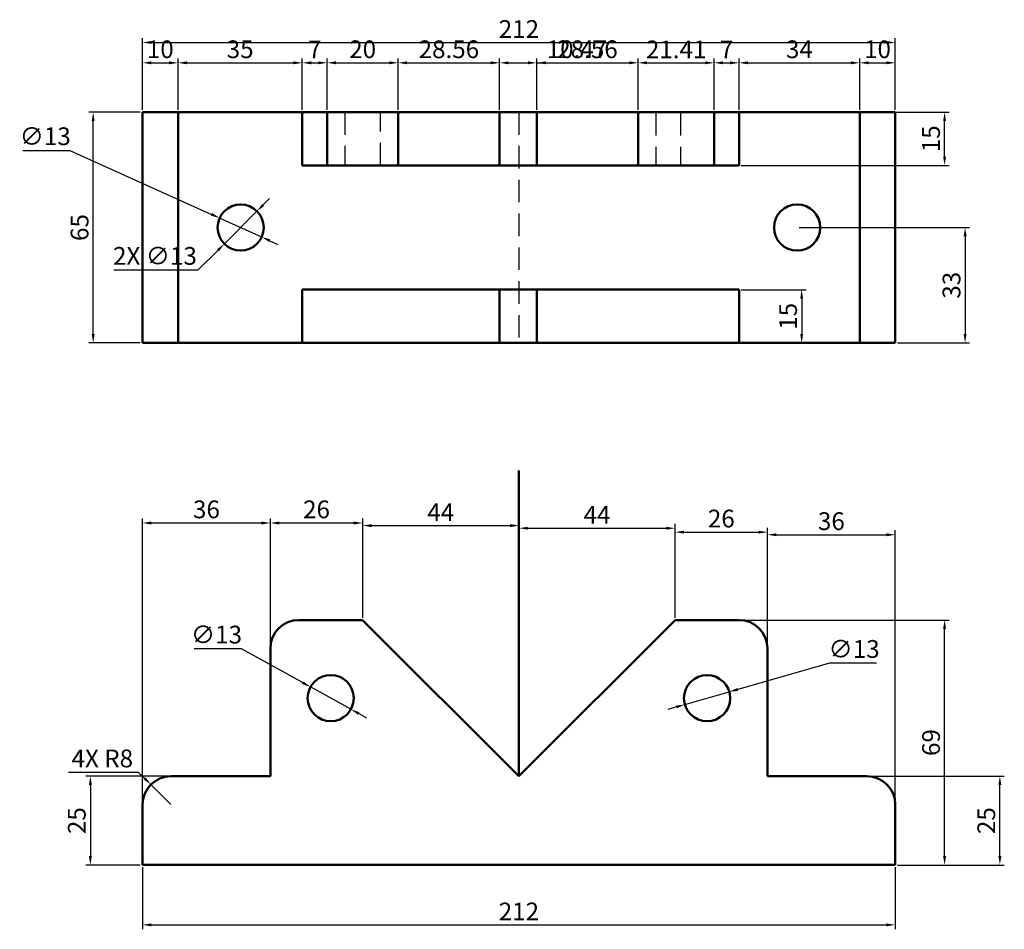
# Model space of a CAD drawing. Units: millimetres. Extents: x 1338 to 1892, y 1867 to 2306.
# Tile 2 of 3: x 1340 to 1617, y 2044 to 2300. Entities that reach past the tile are written whole.
import ezdxf

# ---------------------------------------------------------------- set-up
doc = ezdxf.new("R2010")
doc.units = ezdxf.units.MM
doc.linetypes.add('HIDDEN', pattern=[9.525, 6.35, -3.175])
for name, color, linetype, lineweight in [('M-DIMS', 2, 'Continuous', 25), ('M-HIDN', 4, 'HIDDEN', 25), ('M-OUTL', 7, 'Continuous', 50)]:
    doc.layers.add(name, color=color, linetype=linetype, lineweight=lineweight)
doc.styles.get("Standard").update_dxf_attribs({"font": 'arial.ttf'})
doc.dimstyles.new('ISO-25', dxfattribs={"dimtxt": 5, "dimasz": 2.5, "dimexe": 1.25, "dimexo": 0.625, "dimtad": 1, "dimtoh": 1, "dimdec": 0, "dimtxsty": 'Standard', "dimcen": 2.5, "dimadec": 0, "dimazin": 0, "dimtfac": 1, "dimtdec": 0, "dimtmove": 0, "dimatfit": 3, "dimfxl": 1, "dimarcsym": 0})

# ---------------------------------------------------------------- blocks, each defined once
blk = doc.blocks.new('*D1')
at = {"layer": 'Defpoints', "color": 0, "transparency": 16777216}
for p in [(1586.71, 2293.39), (1374.71, 2273.75), (1586.71, 2273.75)]:
    blk.add_point(p, dxfattribs=at)
at = {"layer": 'M-DIMS', "color": 0, "lineweight": -2, "transparency": 16777216}
for p, q in [((1374.71, 2274.38), (1374.71, 2294.64)), ((1377.21, 2293.39), (1584.21, 2293.39)), ((1586.71, 2274.38), (1586.71, 2294.64))]:
    blk.add_line(p, q, dxfattribs=at)
at = {"layer": 'M-DIMS', "color": 0, "transparency": 16777216}
for points in [[(1377.21, 2293.8), (1377.21, 2292.97), (1374.71, 2293.39)], [(1584.21, 2293.8), (1584.21, 2292.97), (1586.71, 2293.39)]]:
    blk.add_solid(points, dxfattribs=at)
at = {"layer": 'M-DIMS', "color": 0, "transparency": 16777216, "insert": (1480.71, 2296.52), "char_height": 5, "attachment_point": 5}
blk.add_mtext('212', dxfattribs=at)
blk = doc.blocks.new('*D2')
at = {"layer": 'Defpoints', "color": 0, "transparency": 16777216}
for p in [(1559.07, 2241.25), (1586.71, 2208.75), (1606.38, 2208.75)]:
    blk.add_point(p, dxfattribs=at)
at = {"layer": 'M-DIMS', "color": 0, "lineweight": -2, "transparency": 16777216}
for p, q in [((1559.69, 2241.25), (1607.63, 2241.25)), ((1606.38, 2238.75), (1606.38, 2211.25)), ((1587.33, 2208.75), (1607.63, 2208.75))]:
    blk.add_line(p, q, dxfattribs=at)
at = {"layer": 'M-DIMS', "color": 0, "transparency": 16777216}
for points in [[(1605.96, 2238.75), (1606.8, 2238.75), (1606.38, 2241.25)], [(1605.96, 2211.25), (1606.8, 2211.25), (1606.38, 2208.75)]]:
    blk.add_solid(points, dxfattribs=at)
at = {"layer": 'M-DIMS', "color": 0, "transparency": 16777216, "insert": (1603.2, 2225), "char_height": 5, "attachment_point": 5, "rotation": 90}
blk.add_mtext('33', dxfattribs=at)
blk = doc.blocks.new('*D3')
at = {"layer": 'Defpoints', "color": 0, "transparency": 16777216}
for p in [(1396.43, 2243.93), (1408.27, 2238.58)]:
    blk.add_point(p, dxfattribs=at)
at = {"layer": 'M-DIMS', "color": 0, "lineweight": -2, "transparency": 16777216}
for p, q in [((1341.01, 2263), (1354.24, 2263)), ((1354.24, 2263), (1394.15, 2244.96)), ((1408.27, 2238.58), (1396.43, 2243.93)), ((1410.55, 2237.55), (1412.83, 2236.52))]:
    blk.add_line(p, q, dxfattribs=at)
at = {"layer": 'M-DIMS', "color": 0, "transparency": 16777216}
for points in [[(1394.32, 2245.34), (1393.98, 2244.58), (1396.43, 2243.93)], [(1410.72, 2237.93), (1410.38, 2237.17), (1408.27, 2238.58)]]:
    blk.add_solid(points, dxfattribs=at)
at = {"layer": 'M-DIMS', "color": 0, "transparency": 16777216, "insert": (1347.31, 2266.32), "char_height": 5, "attachment_point": 5}
blk.add_mtext('∅13', dxfattribs=at)
blk = doc.blocks.new('*D4')
at = {"layer": 'Defpoints', "color": 0, "transparency": 16777216}
for p in [(1542.71, 2223.75), (1542.71, 2208.75), (1560.35, 2208.75)]:
    blk.add_point(p, dxfattribs=at)
at = {"layer": 'M-DIMS', "color": 0, "lineweight": -2, "transparency": 16777216}
for p, q in [((1543.33, 2223.75), (1561.6, 2223.75)), ((1560.35, 2221.25), (1560.35, 2211.25)), ((1543.33, 2208.75), (1561.6, 2208.75))]:
    blk.add_line(p, q, dxfattribs=at)
at = {"layer": 'M-DIMS', "color": 0, "transparency": 16777216}
for points in [[(1559.93, 2221.25), (1560.77, 2221.25), (1560.35, 2223.75)], [(1559.93, 2211.25), (1560.77, 2211.25), (1560.35, 2208.75)]]:
    blk.add_solid(points, dxfattribs=at)
at = {"layer": 'M-DIMS', "color": 0, "transparency": 16777216, "insert": (1557.17, 2216.25), "char_height": 5, "attachment_point": 5, "rotation": 90}
blk.add_mtext('15', dxfattribs=at)
blk = doc.blocks.new('*D5')
at = {"layer": 'Defpoints', "color": 0, "transparency": 16777216}
for p in [(1374.71, 2061.68), (1586.71, 2061.68), (1586.71, 2044.82)]:
    blk.add_point(p, dxfattribs=at)
at = {"layer": 'M-DIMS', "color": 0, "lineweight": -2, "transparency": 16777216}
for p, q in [((1374.71, 2061.06), (1374.71, 2043.57)), ((1586.71, 2061.06), (1586.71, 2043.57)), ((1377.21, 2044.82), (1584.21, 2044.82))]:
    blk.add_line(p, q, dxfattribs=at)
at = {"layer": 'M-DIMS', "color": 0, "transparency": 16777216}
for points in [[(1377.21, 2045.23), (1377.21, 2044.4), (1374.71, 2044.82)], [(1584.21, 2045.23), (1584.21, 2044.4), (1586.71, 2044.82)]]:
    blk.add_solid(points, dxfattribs=at)
at = {"layer": 'M-DIMS', "color": 0, "transparency": 16777216, "insert": (1480.71, 2047.95), "char_height": 5, "attachment_point": 5}
blk.add_mtext('212', dxfattribs=at)
blk = doc.blocks.new('*D6')
at = {"layer": 'Defpoints', "color": 0, "transparency": 16777216}
for p in [(1382.71, 2086.68), (1360.02, 2061.68), (1374.71, 2061.68)]:
    blk.add_point(p, dxfattribs=at)
at = {"layer": 'M-DIMS', "color": 0, "lineweight": -2, "transparency": 16777216}
for p, q in [((1382.08, 2086.68), (1358.77, 2086.68)), ((1360.02, 2084.18), (1360.02, 2064.18)), ((1374.08, 2061.68), (1358.77, 2061.68))]:
    blk.add_line(p, q, dxfattribs=at)
at = {"layer": 'M-DIMS', "color": 0, "transparency": 16777216}
for points in [[(1359.6, 2084.18), (1360.44, 2084.18), (1360.02, 2086.68)], [(1359.6, 2064.18), (1360.44, 2064.18), (1360.02, 2061.68)]]:
    blk.add_solid(points, dxfattribs=at)
at = {"layer": 'M-DIMS', "color": 0, "transparency": 16777216, "insert": (1356.84, 2074.18), "char_height": 5, "attachment_point": 5, "rotation": 90}
blk.add_mtext('25', dxfattribs=at)
blk = doc.blocks.new('*D7')
at = {"layer": 'Defpoints', "color": 0, "transparency": 16777216}
for p in [(1410.71, 2158.03), (1410.71, 2086.68), (1374.71, 2078.68)]:
    blk.add_point(p, dxfattribs=at)
at = {"layer": 'M-DIMS', "color": 0, "lineweight": -2, "transparency": 16777216}
for p, q in [((1374.71, 2079.31), (1374.71, 2159.28)), ((1377.21, 2158.03), (1408.21, 2158.03)), ((1410.71, 2087.31), (1410.71, 2159.28))]:
    blk.add_line(p, q, dxfattribs=at)
at = {"layer": 'M-DIMS', "color": 0, "transparency": 16777216}
for points in [[(1377.21, 2158.44), (1377.21, 2157.61), (1374.71, 2158.03)], [(1408.21, 2158.44), (1408.21, 2157.61), (1410.71, 2158.03)]]:
    blk.add_solid(points, dxfattribs=at)
at = {"layer": 'M-DIMS', "color": 0, "transparency": 16777216, "insert": (1392.71, 2161.21), "char_height": 5, "attachment_point": 5}
blk.add_mtext('36', dxfattribs=at)
blk = doc.blocks.new('*D8')
at = {"layer": 'Defpoints', "color": 0, "transparency": 16777216}
for p in [(1436.71, 2158.03), (1436.71, 2130.68), (1410.71, 2122.68)]:
    blk.add_point(p, dxfattribs=at)
at = {"layer": 'M-DIMS', "color": 0, "lineweight": -2, "transparency": 16777216}
for p, q in [((1410.71, 2123.31), (1410.71, 2159.28)), ((1413.21, 2158.03), (1434.21, 2158.03)), ((1436.71, 2131.31), (1436.71, 2159.28))]:
    blk.add_line(p, q, dxfattribs=at)
at = {"layer": 'M-DIMS', "color": 0, "transparency": 16777216}
for points in [[(1413.21, 2158.44), (1413.21, 2157.61), (1410.71, 2158.03)], [(1434.21, 2158.44), (1434.21, 2157.61), (1436.71, 2158.03)]]:
    blk.add_solid(points, dxfattribs=at)
at = {"layer": 'M-DIMS', "color": 0, "transparency": 16777216, "insert": (1423.71, 2161.21), "char_height": 5, "attachment_point": 5}
blk.add_mtext('26', dxfattribs=at)
blk = doc.blocks.new('*D9')
at = {"layer": 'Defpoints', "color": 0, "transparency": 16777216}
for p in [(1480.71, 2157.29), (1436.71, 2130.68), (1480.71, 2129.77)]:
    blk.add_point(p, dxfattribs=at)
at = {"layer": 'M-DIMS', "color": 0, "lineweight": -2, "transparency": 16777216}
for p, q in [((1436.71, 2131.31), (1436.71, 2158.54)), ((1480.71, 2130.39), (1480.71, 2158.54)), ((1439.21, 2157.29), (1478.21, 2157.29))]:
    blk.add_line(p, q, dxfattribs=at)
at = {"layer": 'M-DIMS', "color": 0, "transparency": 16777216}
for points in [[(1439.21, 2157.71), (1439.21, 2156.87), (1436.71, 2157.29)], [(1478.21, 2157.71), (1478.21, 2156.87), (1480.71, 2157.29)]]:
    blk.add_solid(points, dxfattribs=at)
at = {"layer": 'M-DIMS', "color": 0, "transparency": 16777216, "insert": (1458.71, 2160.41), "char_height": 5, "attachment_point": 5}
blk.add_mtext('44', dxfattribs=at)
blk = doc.blocks.new('*D10')
at = {"layer": 'Defpoints', "color": 0, "transparency": 16777216}
for p in [(1524.71, 2156.55), (1480.71, 2129.77), (1524.71, 2130.68)]:
    blk.add_point(p, dxfattribs=at)
at = {"layer": 'M-DIMS', "color": 0, "lineweight": -2, "transparency": 16777216}
for p, q in [((1480.71, 2130.39), (1480.71, 2157.8)), ((1524.71, 2131.31), (1524.71, 2157.8)), ((1483.21, 2156.55), (1522.21, 2156.55))]:
    blk.add_line(p, q, dxfattribs=at)
at = {"layer": 'M-DIMS', "color": 0, "transparency": 16777216}
for points in [[(1483.21, 2156.97), (1483.21, 2156.14), (1480.71, 2156.55)], [(1522.21, 2156.97), (1522.21, 2156.14), (1524.71, 2156.55)]]:
    blk.add_solid(points, dxfattribs=at)
at = {"layer": 'M-DIMS', "color": 0, "transparency": 16777216, "insert": (1502.71, 2159.68), "char_height": 5, "attachment_point": 5}
blk.add_mtext('44', dxfattribs=at)
blk = doc.blocks.new('*D11')
at = {"layer": 'Defpoints', "color": 0, "transparency": 16777216}
for p in [(1550.71, 2155.45), (1524.71, 2130.68), (1550.71, 2122.68)]:
    blk.add_point(p, dxfattribs=at)
at = {"layer": 'M-DIMS', "color": 0, "lineweight": -2, "transparency": 16777216}
for p, q in [((1524.71, 2131.31), (1524.71, 2156.7)), ((1527.21, 2155.45), (1548.21, 2155.45)), ((1550.71, 2123.31), (1550.71, 2156.7))]:
    blk.add_line(p, q, dxfattribs=at)
at = {"layer": 'M-DIMS', "color": 0, "transparency": 16777216}
for points in [[(1527.21, 2155.86), (1527.21, 2155.03), (1524.71, 2155.45)], [(1548.21, 2155.86), (1548.21, 2155.03), (1550.71, 2155.45)]]:
    blk.add_solid(points, dxfattribs=at)
at = {"layer": 'M-DIMS', "color": 0, "transparency": 16777216, "insert": (1537.71, 2158.62), "char_height": 5, "attachment_point": 5}
blk.add_mtext('26', dxfattribs=at)
blk = doc.blocks.new('*D12')
at = {"layer": 'Defpoints', "color": 0, "transparency": 16777216}
for p in [(1586.71, 2154.71), (1550.71, 2104.68), (1586.71, 2078.68)]:
    blk.add_point(p, dxfattribs=at)
at = {"layer": 'M-DIMS', "color": 0, "lineweight": -2, "transparency": 16777216}
for p, q in [((1550.71, 2105.31), (1550.71, 2155.96)), ((1553.21, 2154.71), (1584.21, 2154.71)), ((1586.71, 2079.31), (1586.71, 2155.96))]:
    blk.add_line(p, q, dxfattribs=at)
at = {"layer": 'M-DIMS', "color": 0, "transparency": 16777216}
for points in [[(1553.21, 2155.13), (1553.21, 2154.29), (1550.71, 2154.71)], [(1584.21, 2155.13), (1584.21, 2154.29), (1586.71, 2154.71)]]:
    blk.add_solid(points, dxfattribs=at)
at = {"layer": 'M-DIMS', "color": 0, "transparency": 16777216, "insert": (1568.71, 2157.89), "char_height": 5, "attachment_point": 5}
blk.add_mtext('36', dxfattribs=at)
blk = doc.blocks.new('*D13')
at = {"layer": 'Defpoints', "color": 0, "transparency": 16777216}
for p in [(1578.71, 2086.68), (1616.17, 2086.68), (1586.71, 2061.68)]:
    blk.add_point(p, dxfattribs=at)
at = {"layer": 'M-DIMS', "color": 0, "lineweight": -2, "transparency": 16777216}
for p, q in [((1579.33, 2086.68), (1617.42, 2086.68)), ((1616.17, 2064.18), (1616.17, 2084.18)), ((1587.33, 2061.68), (1617.42, 2061.68))]:
    blk.add_line(p, q, dxfattribs=at)
at = {"layer": 'M-DIMS', "color": 0, "transparency": 16777216}
for points in [[(1615.75, 2084.18), (1616.59, 2084.18), (1616.17, 2086.68)], [(1615.75, 2064.18), (1616.59, 2064.18), (1616.17, 2061.68)]]:
    blk.add_solid(points, dxfattribs=at)
at = {"layer": 'M-DIMS', "color": 0, "transparency": 16777216, "insert": (1612.99, 2074.18), "char_height": 5, "attachment_point": 5, "rotation": 90}
blk.add_mtext('25', dxfattribs=at)
blk = doc.blocks.new('*D14')
at = {"layer": 'Defpoints', "color": 0, "transparency": 16777216}
for p in [(1539.96, 2110.47), (1527.46, 2106.89)]:
    blk.add_point(p, dxfattribs=at)
at = {"layer": 'M-DIMS', "color": 0, "lineweight": -2, "transparency": 16777216}
for p, q in [((1568.19, 2118.57), (1542.36, 2111.16)), ((1581.41, 2118.57), (1568.19, 2118.57)), ((1527.46, 2106.89), (1539.96, 2110.47)), ((1525.06, 2106.2), (1522.65, 2105.51))]:
    blk.add_line(p, q, dxfattribs=at)
at = {"layer": 'M-DIMS', "color": 0, "transparency": 16777216}
for points in [[(1542.24, 2111.56), (1542.47, 2110.76), (1539.96, 2110.47)], [(1524.94, 2106.6), (1525.17, 2105.8), (1527.46, 2106.89)]]:
    blk.add_solid(points, dxfattribs=at)
at = {"layer": 'M-DIMS', "color": 0, "transparency": 16777216, "insert": (1575.11, 2121.89), "char_height": 5, "attachment_point": 5}
blk.add_mtext('∅13', dxfattribs=at)
blk = doc.blocks.new('*D15')
at = {"layer": 'Defpoints', "color": 0, "transparency": 16777216}
for p in [(1422.02, 2111.84), (1433.4, 2105.56)]:
    blk.add_point(p, dxfattribs=at)
at = {"layer": 'M-DIMS', "color": 0, "lineweight": -2, "transparency": 16777216}
for p, q in [((1389.24, 2122.63), (1402.47, 2122.63)), ((1402.47, 2122.63), (1419.83, 2113.05)), ((1433.4, 2105.56), (1422.02, 2111.84)), ((1435.59, 2104.36), (1437.78, 2103.15))]:
    blk.add_line(p, q, dxfattribs=at)
at = {"layer": 'M-DIMS', "color": 0, "transparency": 16777216}
for points in [[(1420.03, 2113.41), (1419.63, 2112.68), (1422.02, 2111.84)], [(1435.79, 2104.72), (1435.39, 2103.99), (1433.4, 2105.56)]]:
    blk.add_solid(points, dxfattribs=at)
at = {"layer": 'M-DIMS', "color": 0, "transparency": 16777216, "insert": (1395.54, 2125.94), "char_height": 5, "attachment_point": 5}
blk.add_mtext('∅13', dxfattribs=at)
blk = doc.blocks.new('*D43')
at = {"layer": 'Defpoints', "color": 0, "transparency": 16777216}
for p in [(1360.81, 2273.75), (1374.71, 2273.75), (1374.71, 2208.75)]:
    blk.add_point(p, dxfattribs=at)
at = {"layer": 'M-DIMS', "color": 0, "lineweight": -2, "transparency": 16777216}
for p, q in [((1374.08, 2273.75), (1359.56, 2273.75)), ((1360.81, 2211.25), (1360.81, 2271.25)), ((1374.08, 2208.75), (1359.56, 2208.75))]:
    blk.add_line(p, q, dxfattribs=at)
at = {"layer": 'M-DIMS', "color": 0, "transparency": 16777216}
for points in [[(1360.39, 2271.25), (1361.22, 2271.25), (1360.81, 2273.75)], [(1360.39, 2211.25), (1361.22, 2211.25), (1360.81, 2208.75)]]:
    blk.add_solid(points, dxfattribs=at)
at = {"layer": 'M-DIMS', "color": 0, "transparency": 16777216, "insert": (1357.63, 2241.25), "char_height": 5, "attachment_point": 5, "rotation": 90}
blk.add_mtext('65', dxfattribs=at)
blk = doc.blocks.new('*D44')
at = {"layer": 'Defpoints', "color": 0, "transparency": 16777216}
for p in [(1384.71, 2287.65), (1374.71, 2273.75), (1384.71, 2273.75)]:
    blk.add_point(p, dxfattribs=at)
at = {"layer": 'M-DIMS', "color": 0, "lineweight": -2, "transparency": 16777216}
for p, q in [((1374.71, 2274.38), (1374.71, 2288.9)), ((1384.71, 2274.38), (1384.71, 2288.9)), ((1377.21, 2287.65), (1382.21, 2287.65))]:
    blk.add_line(p, q, dxfattribs=at)
at = {"layer": 'M-DIMS', "color": 0, "transparency": 16777216}
for points in [[(1377.21, 2288.07), (1377.21, 2287.24), (1374.71, 2287.65)], [(1382.21, 2288.07), (1382.21, 2287.24), (1384.71, 2287.65)]]:
    blk.add_solid(points, dxfattribs=at)
at = {"layer": 'M-DIMS', "color": 0, "transparency": 16777216, "insert": (1379.71, 2290.83), "char_height": 5, "attachment_point": 5}
blk.add_mtext('10', dxfattribs=at)
blk = doc.blocks.new('*D45')
at = {"layer": 'Defpoints', "color": 0, "transparency": 16777216}
for p in [(1586.71, 2287.65), (1576.71, 2273.75), (1586.71, 2273.75)]:
    blk.add_point(p, dxfattribs=at)
at = {"layer": 'M-DIMS', "color": 0, "lineweight": -2, "transparency": 16777216}
for p, q in [((1576.71, 2274.38), (1576.71, 2288.9)), ((1586.71, 2274.38), (1586.71, 2288.9)), ((1579.21, 2287.65), (1584.21, 2287.65))]:
    blk.add_line(p, q, dxfattribs=at)
at = {"layer": 'M-DIMS', "color": 0, "transparency": 16777216}
for points in [[(1579.21, 2288.07), (1579.21, 2287.24), (1576.71, 2287.65)], [(1584.21, 2288.07), (1584.21, 2287.24), (1586.71, 2287.65)]]:
    blk.add_solid(points, dxfattribs=at)
at = {"layer": 'M-DIMS', "color": 0, "transparency": 16777216, "insert": (1581.71, 2290.83), "char_height": 5, "attachment_point": 5}
blk.add_mtext('10', dxfattribs=at)
blk = doc.blocks.new('*D46')
at = {"layer": 'Defpoints', "color": 0, "transparency": 16777216}
for p in [(1419.71, 2287.65), (1384.71, 2273.75), (1419.71, 2273.75)]:
    blk.add_point(p, dxfattribs=at)
at = {"layer": 'M-DIMS', "color": 0, "lineweight": -2, "transparency": 16777216}
for p, q in [((1384.71, 2274.38), (1384.71, 2288.9)), ((1419.71, 2274.38), (1419.71, 2288.9)), ((1387.21, 2287.65), (1417.21, 2287.65))]:
    blk.add_line(p, q, dxfattribs=at)
at = {"layer": 'M-DIMS', "color": 0, "transparency": 16777216}
for points in [[(1387.21, 2288.07), (1387.21, 2287.24), (1384.71, 2287.65)], [(1417.21, 2288.07), (1417.21, 2287.24), (1419.71, 2287.65)]]:
    blk.add_solid(points, dxfattribs=at)
at = {"layer": 'M-DIMS', "color": 0, "transparency": 16777216, "insert": (1402.21, 2290.83), "char_height": 5, "attachment_point": 5}
blk.add_mtext('35', dxfattribs=at)
blk = doc.blocks.new('*D47')
at = {"layer": 'Defpoints', "color": 0, "transparency": 16777216}
for p in [(1576.71, 2287.65), (1542.71, 2273.75), (1576.71, 2273.75)]:
    blk.add_point(p, dxfattribs=at)
at = {"layer": 'M-DIMS', "color": 0, "lineweight": -2, "transparency": 16777216}
for p, q in [((1542.71, 2274.38), (1542.71, 2288.9)), ((1576.71, 2274.38), (1576.71, 2288.9)), ((1545.21, 2287.65), (1574.21, 2287.65))]:
    blk.add_line(p, q, dxfattribs=at)
at = {"layer": 'M-DIMS', "color": 0, "transparency": 16777216}
for points in [[(1545.21, 2288.07), (1545.21, 2287.24), (1542.71, 2287.65)], [(1574.21, 2288.07), (1574.21, 2287.24), (1576.71, 2287.65)]]:
    blk.add_solid(points, dxfattribs=at)
at = {"layer": 'M-DIMS', "color": 0, "transparency": 16777216, "insert": (1559.71, 2290.83), "char_height": 5, "attachment_point": 5}
blk.add_mtext('34', dxfattribs=at)
blk = doc.blocks.new('*D48')
at = {"layer": 'Defpoints', "color": 0, "transparency": 16777216}
for p in [(1426.71, 2287.65), (1419.71, 2273.75), (1426.71, 2273.75)]:
    blk.add_point(p, dxfattribs=at)
at = {"layer": 'M-DIMS', "color": 0, "lineweight": -2, "transparency": 16777216}
for p, q in [((1419.71, 2274.38), (1419.71, 2288.9)), ((1426.71, 2274.38), (1426.71, 2288.9)), ((1422.21, 2287.65), (1424.21, 2287.65))]:
    blk.add_line(p, q, dxfattribs=at)
at = {"layer": 'M-DIMS', "color": 0, "transparency": 16777216}
for points in [[(1422.21, 2288.07), (1422.21, 2287.24), (1419.71, 2287.65)], [(1424.21, 2288.07), (1424.21, 2287.24), (1426.71, 2287.65)]]:
    blk.add_solid(points, dxfattribs=at)
at = {"layer": 'M-DIMS', "color": 0, "transparency": 16777216, "insert": (1423.21, 2290.78), "char_height": 5, "attachment_point": 5}
blk.add_mtext('7', dxfattribs=at)
blk = doc.blocks.new('*D49')
at = {"layer": 'Defpoints', "color": 0, "transparency": 16777216}
for p in [(1446.71, 2287.65), (1426.71, 2273.75), (1446.71, 2273.75)]:
    blk.add_point(p, dxfattribs=at)
at = {"layer": 'M-DIMS', "color": 0, "lineweight": -2, "transparency": 16777216}
for p, q in [((1426.71, 2274.38), (1426.71, 2288.9)), ((1446.71, 2274.38), (1446.71, 2288.9)), ((1429.21, 2287.65), (1444.21, 2287.65))]:
    blk.add_line(p, q, dxfattribs=at)
at = {"layer": 'M-DIMS', "color": 0, "transparency": 16777216}
for points in [[(1429.21, 2288.07), (1429.21, 2287.24), (1426.71, 2287.65)], [(1444.21, 2288.07), (1444.21, 2287.24), (1446.71, 2287.65)]]:
    blk.add_solid(points, dxfattribs=at)
at = {"layer": 'M-DIMS', "color": 0, "transparency": 16777216, "insert": (1436.71, 2290.83), "char_height": 5, "attachment_point": 5}
blk.add_mtext('20', dxfattribs=at)
blk = doc.blocks.new('*D50')
at = {"layer": 'Defpoints', "color": 0, "transparency": 16777216}
for p in [(1475.27, 2287.65), (1446.71, 2273.75), (1475.27, 2273.75)]:
    blk.add_point(p, dxfattribs=at)
at = {"layer": 'M-DIMS', "color": 0, "lineweight": -2, "transparency": 16777216}
for p, q in [((1446.71, 2274.38), (1446.71, 2288.9)), ((1475.27, 2274.38), (1475.27, 2288.9)), ((1449.21, 2287.65), (1472.77, 2287.65))]:
    blk.add_line(p, q, dxfattribs=at)
at = {"layer": 'M-DIMS', "color": 0, "transparency": 16777216}
for points in [[(1449.21, 2288.07), (1449.21, 2287.24), (1446.71, 2287.65)], [(1472.77, 2288.07), (1472.77, 2287.24), (1475.27, 2287.65)]]:
    blk.add_solid(points, dxfattribs=at)
at = {"layer": 'M-DIMS', "color": 0, "transparency": 16777216, "insert": (1460.99, 2290.83), "char_height": 5, "attachment_point": 5}
blk.add_mtext('28.56', dxfattribs=at)
blk = doc.blocks.new('*D51')
at = {"layer": 'Defpoints', "color": 0, "transparency": 16777216}
for p in [(1485.74, 2287.65), (1475.27, 2273.75), (1485.74, 2273.75)]:
    blk.add_point(p, dxfattribs=at)
at = {"layer": 'M-DIMS', "color": 0, "lineweight": -2, "transparency": 16777216}
for p, q in [((1475.27, 2274.38), (1475.27, 2288.9)), ((1485.74, 2274.38), (1485.74, 2288.9)), ((1477.77, 2287.65), (1483.24, 2287.65)), ((1485.74, 2287.65), (1505.89, 2287.65))]:
    blk.add_line(p, q, dxfattribs=at)
at = {"layer": 'M-DIMS', "color": 0, "transparency": 16777216}
for points in [[(1477.77, 2288.07), (1477.77, 2287.24), (1475.27, 2287.65)], [(1483.24, 2288.07), (1483.24, 2287.24), (1485.74, 2287.65)]]:
    blk.add_solid(points, dxfattribs=at)
at = {"layer": 'M-DIMS', "color": 0, "transparency": 16777216, "insert": (1497.06, 2290.83), "char_height": 5, "attachment_point": 5}
blk.add_mtext('10.47', dxfattribs=at)
blk = doc.blocks.new('*D52')
at = {"layer": 'Defpoints', "color": 0, "transparency": 16777216}
for p in [(1514.3, 2287.65), (1485.74, 2273.75), (1514.3, 2273.75)]:
    blk.add_point(p, dxfattribs=at)
at = {"layer": 'M-DIMS', "color": 0, "lineweight": -2, "transparency": 16777216}
for p, q in [((1485.74, 2274.38), (1485.74, 2288.9)), ((1514.3, 2274.38), (1514.3, 2288.9)), ((1488.24, 2287.65), (1511.8, 2287.65))]:
    blk.add_line(p, q, dxfattribs=at)
at = {"layer": 'M-DIMS', "color": 0, "transparency": 16777216}
for points in [[(1488.24, 2288.07), (1488.24, 2287.24), (1485.74, 2287.65)], [(1511.8, 2288.07), (1511.8, 2287.24), (1514.3, 2287.65)]]:
    blk.add_solid(points, dxfattribs=at)
at = {"layer": 'M-DIMS', "color": 0, "transparency": 16777216, "insert": (1500.02, 2290.83), "char_height": 5, "attachment_point": 5}
blk.add_mtext('28.56', dxfattribs=at)
blk = doc.blocks.new('*D53')
at = {"layer": 'Defpoints', "color": 0, "transparency": 16777216}
for p in [(1535.71, 2287.65), (1514.3, 2273.75), (1535.71, 2273.75)]:
    blk.add_point(p, dxfattribs=at)
at = {"layer": 'M-DIMS', "color": 0, "lineweight": -2, "transparency": 16777216}
for p, q in [((1514.3, 2274.38), (1514.3, 2288.9)), ((1535.71, 2274.38), (1535.71, 2288.9)), ((1516.8, 2287.65), (1533.21, 2287.65))]:
    blk.add_line(p, q, dxfattribs=at)
at = {"layer": 'M-DIMS', "color": 0, "transparency": 16777216}
for points in [[(1516.8, 2288.07), (1516.8, 2287.24), (1514.3, 2287.65)], [(1533.21, 2288.07), (1533.21, 2287.24), (1535.71, 2287.65)]]:
    blk.add_solid(points, dxfattribs=at)
at = {"layer": 'M-DIMS', "color": 0, "transparency": 16777216, "insert": (1525, 2290.79), "char_height": 5, "attachment_point": 5}
blk.add_mtext('21.41', dxfattribs=at)
blk = doc.blocks.new('*D54')
at = {"layer": 'Defpoints', "color": 0, "transparency": 16777216}
for p in [(1542.71, 2287.65), (1535.71, 2273.75), (1542.71, 2273.75)]:
    blk.add_point(p, dxfattribs=at)
at = {"layer": 'M-DIMS', "color": 0, "lineweight": -2, "transparency": 16777216}
for p, q in [((1535.71, 2274.38), (1535.71, 2288.9)), ((1542.71, 2274.38), (1542.71, 2288.9)), ((1538.21, 2287.65), (1540.21, 2287.65))]:
    blk.add_line(p, q, dxfattribs=at)
at = {"layer": 'M-DIMS', "color": 0, "transparency": 16777216}
for points in [[(1538.21, 2288.07), (1538.21, 2287.24), (1535.71, 2287.65)], [(1540.21, 2288.07), (1540.21, 2287.24), (1542.71, 2287.65)]]:
    blk.add_solid(points, dxfattribs=at)
at = {"layer": 'M-DIMS', "color": 0, "transparency": 16777216, "insert": (1539.21, 2290.78), "char_height": 5, "attachment_point": 5}
blk.add_mtext('7', dxfattribs=at)
blk = doc.blocks.new('*D55')
at = {"layer": 'Defpoints', "color": 0, "transparency": 16777216}
for p in [(1542.71, 2273.75), (1600.61, 2273.75), (1542.71, 2258.75)]:
    blk.add_point(p, dxfattribs=at)
at = {"layer": 'M-DIMS', "color": 0, "lineweight": -2, "transparency": 16777216}
for p, q in [((1543.33, 2273.75), (1601.86, 2273.75)), ((1600.61, 2261.25), (1600.61, 2271.25)), ((1543.33, 2258.75), (1601.86, 2258.75))]:
    blk.add_line(p, q, dxfattribs=at)
at = {"layer": 'M-DIMS', "color": 0, "transparency": 16777216}
for points in [[(1600.19, 2271.25), (1601.02, 2271.25), (1600.61, 2273.75)], [(1600.19, 2261.25), (1601.02, 2261.25), (1600.61, 2258.75)]]:
    blk.add_solid(points, dxfattribs=at)
at = {"layer": 'M-DIMS', "color": 0, "transparency": 16777216, "insert": (1597.43, 2266.25), "char_height": 5, "attachment_point": 5, "rotation": 90}
blk.add_mtext('15', dxfattribs=at)
blk = doc.blocks.new('*D56')
at = {"layer": 'Defpoints', "color": 0, "transparency": 16777216}
for p in [(1542.71, 2130.68), (1600.61, 2130.68), (1586.71, 2061.68)]:
    blk.add_point(p, dxfattribs=at)
at = {"layer": 'M-DIMS', "color": 0, "lineweight": -2, "transparency": 16777216}
for p, q in [((1543.33, 2130.68), (1601.86, 2130.68)), ((1600.61, 2064.18), (1600.61, 2128.18)), ((1587.33, 2061.68), (1601.86, 2061.68))]:
    blk.add_line(p, q, dxfattribs=at)
at = {"layer": 'M-DIMS', "color": 0, "transparency": 16777216}
for points in [[(1600.19, 2128.18), (1601.02, 2128.18), (1600.61, 2130.68)], [(1600.19, 2064.18), (1601.02, 2064.18), (1600.61, 2061.68)]]:
    blk.add_solid(points, dxfattribs=at)
at = {"layer": 'M-DIMS', "color": 0, "transparency": 16777216, "insert": (1597.43, 2096.18), "char_height": 5, "attachment_point": 5, "rotation": 90}
blk.add_mtext('69', dxfattribs=at)
blk = doc.blocks.new('*D72')
at = {"layer": 'Defpoints', "color": 0, "transparency": 16777216}
for p in [(1406.94, 2245.85), (1397.75, 2236.65)]:
    blk.add_point(p, dxfattribs=at)
at = {"layer": 'M-DIMS', "color": 0, "lineweight": -2, "transparency": 16777216}
for p, q in [((1408.71, 2247.62), (1410.48, 2249.39)), ((1406.94, 2245.85), (1397.75, 2236.65)), ((1390.42, 2229.31), (1395.99, 2234.89)), ((1366.63, 2229.31), (1390.42, 2229.31))]:
    blk.add_line(p, q, dxfattribs=at)
at = {"layer": 'M-DIMS', "color": 0, "transparency": 16777216}
for points in [[(1408.41, 2247.92), (1409, 2247.33), (1406.94, 2245.85)], [(1395.69, 2235.18), (1396.28, 2234.59), (1397.75, 2236.65)]]:
    blk.add_solid(points, dxfattribs=at)
at = {"layer": 'M-DIMS', "color": 0, "transparency": 16777216, "insert": (1378.21, 2232.62), "char_height": 5, "attachment_point": 5}
blk.add_mtext('2X ∅13', dxfattribs=at)
blk = doc.blocks.new('*D73')
at = {"layer": 'Defpoints', "color": 0, "transparency": 16777216}
for p in [(1377.05, 2084.34), (1382.71, 2078.68)]:
    blk.add_point(p, dxfattribs=at)
at = {"layer": 'M-DIMS', "color": 0, "lineweight": -2, "transparency": 16777216}
for p, q in [((1353.87, 2087.88), (1373.52, 2087.88)), ((1373.52, 2087.88), (1375.28, 2086.11)), ((1382.71, 2078.68), (1377.05, 2084.34))]:
    blk.add_line(p, q, dxfattribs=at)
at = {"layer": 'M-DIMS', "color": 0, "transparency": 16777216}
blk.add_solid([(1375.58, 2086.4), (1374.99, 2085.81), (1377.05, 2084.34)], dxfattribs=at)
at = {"layer": 'M-DIMS', "color": 0, "transparency": 16777216, "insert": (1363.38, 2091.05), "char_height": 5, "attachment_point": 5}
blk.add_mtext('4X R8', dxfattribs=at)

msp = doc.modelspace()

# ---------------------------------------------------------------- linework, layer by layer
at = {"layer": 'M-HIDN'}
for p, q in [((1426.708, 2273.754), (1431.708, 2273.754)), ((1431.708, 2273.754), (1431.708, 2258.754)), ((1441.708, 2258.754), (1441.708, 2273.754)), ((1480.708, 2273.754), (1480.708, 2208.754)), ((1519.298, 2273.487), (1519.298, 2258.754)), ((1526.243, 2273.487), (1526.243, 2258.754))]:
    msp.add_line(p, q, dxfattribs=at)
at = {"layer": 'M-OUTL'}
for p, q in [((1374.708, 2273.754), (1586.708, 2273.754)), ((1374.708, 2208.754), (1374.708, 2273.754)), ((1374.708, 2273.754), (1384.708, 2273.754)), ((1374.708, 2273.754), (1374.708, 2273.754)), ((1374.708, 2273.754), (1419.708, 2273.754)), ((1384.708, 2273.754), (1384.708, 2208.754)), ((1419.708, 2273.754), (1419.708, 2258.754)), ((1419.708, 2273.754), (1419.708, 2273.754)), ((1419.708, 2273.754), (1426.708, 2273.754)), ((1426.708, 2273.754), (1426.708, 2258.754)), ((1446.708, 2273.754), (1446.708, 2258.754)), ((1475.268, 2273.754), (1475.268, 2258.754)), ((1485.738, 2273.754), (1485.738, 2258.754)), ((1514.298, 2266.254), (1514.298, 2273.754)), ((1519.298, 2273.487), (1519.298, 2273.754)), ((1542.708, 2273.754), (1535.708, 2273.754)), ((1535.708, 2273.754), (1535.708, 2258.754)), ((1542.708, 2258.754), (1542.708, 2273.754)), ((1586.708, 2273.754), (1576.708, 2273.754)), ((1576.708, 2273.754), (1576.708, 2208.754)), ((1586.708, 2273.754), (1586.708, 2208.754)), ((1514.298, 2266.254), (1514.298, 2258.754)), ((1419.708, 2258.754), (1542.708, 2258.754)), ((1419.708, 2208.754), (1419.708, 2223.754)), ((1419.708, 2223.754), (1542.708, 2223.754)), ((1475.268, 2223.754), (1475.268, 2208.754)), ((1485.738, 2223.754), (1485.738, 2208.754)), ((1542.708, 2208.754), (1542.708, 2223.754)), ((1586.708, 2208.754), (1374.708, 2208.754)), ((1480.708, 2086.683), (1480.708, 2172.852)), ((1418.708, 2130.683), (1436.708, 2130.683)), ((1480.708, 2086.683), (1436.708, 2130.683)), ((1480.708, 2086.683), (1524.708, 2130.683)), ((1542.708, 2130.683), (1524.708, 2130.683)), ((1410.708, 2086.683), (1410.708, 2122.683)), ((1550.708, 2086.683), (1550.708, 2122.683)), ((1382.708, 2086.683), (1410.708, 2086.683)), ((1578.708, 2086.683), (1550.708, 2086.683)), ((1374.708, 2078.683), (1374.708, 2061.683)), ((1374.708, 2061.683), (1374.708, 2078.683)), ((1586.708, 2061.683), (1586.708, 2078.683)), ((1374.708, 2061.683), (1586.708, 2061.683))]:
    msp.add_line(p, q, dxfattribs=at)
for centre in [(1402.348, 2241.254), (1559.068, 2241.254), (1427.708, 2108.702), (1533.708, 2108.683)]:
    msp.add_circle(centre, 6.5, dxfattribs=at)
for centre, start, end in [((1418.708, 2122.683), 90, 180), ((1542.708, 2122.683), 0, 90), ((1382.708, 2078.683), 90, 180), ((1578.708, 2078.683), 0, 90)]:
    msp.add_arc(centre, 8, start, end, dxfattribs=at)

# ---------------------------------------------------------------- dimensions: what is measured, and where the dimension line sits
at = {"layer": 'M-DIMS'}
for base, p1, p2, override, picture, middle in [((1586.708, 2293.387), (1374.708, 2273.754), (1586.708, 2273.754), {"dimclrd": 0, "dimclre": 0, "dimclrt": 0}, '*D1', (1480.708, 2296.522)), ((1384.708, 2287.654), (1374.708, 2273.754), (1384.708, 2273.754), {"dimdec": 0, "dimlfac": 1, "dimrnd": 0, "dimzin": 0, "dimdsep": 46, "dimlunit": 2}, '*D44', (1379.708, 2290.832)), ((1419.708, 2287.654), (1384.708, 2273.754), (1419.708, 2273.754), {"dimdec": 0, "dimlfac": 1, "dimrnd": 0, "dimzin": 0, "dimdsep": 46, "dimlunit": 2}, '*D46', (1402.208, 2290.833)), ((1426.708, 2287.654), (1419.708, 2273.754), (1426.708, 2273.754), {"dimdec": 0, "dimlfac": 1, "dimrnd": 0, "dimzin": 0, "dimdsep": 46, "dimlunit": 2}, '*D48', (1423.208, 2290.779)), ((1446.708, 2287.654), (1426.708, 2273.754), (1446.708, 2273.754), {"dimdec": 0, "dimlfac": 1, "dimrnd": 0, "dimzin": 0, "dimdsep": 46, "dimlunit": 2}, '*D49', (1436.708, 2290.832)), ((1475.268, 2287.654), (1446.708, 2273.754), (1475.268, 2273.754), {"dimdec": 2, "dimlfac": 1, "dimrnd": 0, "dimzin": 0, "dimdsep": 46, "dimlunit": 2}, '*D50', (1460.988, 2290.832)), ((1485.738, 2287.654), (1475.268, 2273.754), (1485.738, 2273.754), {"dimdec": 2, "dimlfac": 1, "dimrnd": 0, "dimzin": 0, "dimdsep": 46, "dimlunit": 2}, '*D51', (1497.063, 2290.832)), ((1514.298, 2287.654), (1485.738, 2273.754), (1514.298, 2273.754), {"dimdec": 2, "dimlfac": 1, "dimrnd": 0, "dimzin": 0, "dimdsep": 46, "dimlunit": 2}, '*D52', (1500.018, 2290.832)), ((1535.708, 2287.654), (1514.298, 2273.754), (1535.708, 2273.754), {"dimdec": 2, "dimlfac": 1, "dimrnd": 0, "dimzin": 0, "dimdsep": 46, "dimlunit": 2}, '*D53', (1525.003, 2290.789)), ((1542.708, 2287.654), (1535.708, 2273.754), (1542.708, 2273.754), {"dimdec": 0, "dimlfac": 1, "dimrnd": 0, "dimzin": 0, "dimdsep": 46, "dimlunit": 2}, '*D54', (1539.208, 2290.779)), ((1576.708, 2287.654), (1542.708, 2273.754), (1576.708, 2273.754), {"dimdec": 0, "dimlfac": 1, "dimrnd": 0, "dimzin": 0, "dimdsep": 46, "dimlunit": 2}, '*D47', (1559.708, 2290.833)), ((1586.708, 2287.654), (1576.708, 2273.754), (1586.708, 2273.754), {"dimdec": 0, "dimlfac": 1, "dimrnd": 0, "dimzin": 0, "dimdsep": 46, "dimlunit": 2}, '*D45', (1581.708, 2290.832)), ((1410.708, 2158.027), (1374.708, 2078.683), (1410.708, 2086.683), {"dimclrd": 0, "dimclre": 0, "dimclrt": 0}, '*D7', (1392.708, 2161.207)), ((1436.708, 2158.027), (1410.708, 2122.683), (1436.708, 2130.683), {"dimclrd": 0, "dimclre": 0, "dimclrt": 0}, '*D8', (1423.708, 2161.205)), ((1480.708, 2157.29), (1436.708, 2130.683), (1480.708, 2129.767), {"dimclrd": 0, "dimclre": 0, "dimclrt": 0}, '*D9', (1458.708, 2160.415)), ((1524.708, 2156.552), (1480.708, 2129.767), (1524.708, 2130.683), {"dimclrd": 0, "dimclre": 0, "dimclrt": 0}, '*D10', (1502.708, 2159.677)), ((1550.708, 2155.446), (1524.708, 2130.683), (1550.708, 2122.683), {"dimclrd": 0, "dimclre": 0, "dimclrt": 0}, '*D11', (1537.708, 2158.624)), ((1586.708, 2154.709), (1550.708, 2104.683), (1586.708, 2078.683), {"dimclrd": 0, "dimclre": 0, "dimclrt": 0}, '*D12', (1568.708, 2157.888)), ((1586.708, 2044.816), (1374.708, 2061.683), (1586.708, 2061.683), {"dimclrd": 0, "dimclre": 0, "dimclrt": 0}, '*D5', (1480.708, 2047.952))]:
    dim = msp.add_linear_dim(base=base, p1=p1, p2=p2, dimstyle='ISO-25', override=override, dxfattribs=at)
    dim.commit()
    dim.dimension.update_dxf_attribs({"geometry": picture, "text_midpoint": middle})
for base, p1, p2, override, picture, middle in [((1360.808, 2273.754), (1374.708, 2208.754), (1374.708, 2273.754), {"dimdec": 0, "dimlfac": 1, "dimrnd": 0, "dimzin": 0, "dimdsep": 46, "dimlunit": 2}, '*D43', (1357.63, 2241.254)), ((1600.608, 2273.754), (1542.708, 2258.754), (1542.708, 2273.754), {"dimdec": 0, "dimlfac": 1, "dimrnd": 0, "dimzin": 0, "dimdsep": 46, "dimlunit": 2}, '*D55', (1597.43, 2266.254)), ((1606.380515165, 2208.753763677), (1559.067980663, 2241.253763677), (1586.707980663, 2208.753763677), {"dimclrd": 0, "dimclre": 0, "dimclrt": 0}, '*D2', (1603.200944906, 2225.003763677)), ((1560.349, 2208.754), (1542.708, 2223.754), (1542.708, 2208.754), {"dimclrd": 0, "dimclre": 0, "dimclrt": 0}, '*D4', (1557.171, 2216.254)), ((1600.608, 2130.683), (1586.708, 2061.683), (1542.708, 2130.683), {"dimdec": 0, "dimlfac": 1, "dimrnd": 0, "dimzin": 0, "dimdsep": 46, "dimlunit": 2}, '*D56', (1597.43, 2096.183)), ((1360.022, 2061.683), (1382.708, 2086.683), (1374.708, 2061.683), {"dimclrd": 0, "dimclre": 0, "dimclrt": 0}, '*D6', (1356.844, 2074.183)), ((1616.169, 2086.683), (1586.708, 2061.683), (1578.708, 2086.683), {"dimclrd": 0, "dimclre": 0, "dimclrt": 0}, '*D13', (1612.991, 2074.183))]:
    dim = msp.add_linear_dim(base=base, p1=p1, p2=p2, angle=90, dimstyle='ISO-25', override=override, dxfattribs=at)
    dim.commit()
    dim.dimension.update_dxf_attribs({"geometry": picture, "text_midpoint": middle})
for p1, p2, picture, middle in [((1408.272, 2238.577), (1396.425, 2243.931), '*D3', (1347.311, 2263)), ((1433.399, 2105.563), (1422.016, 2111.842), '*D15', (1395.541, 2122.626)), ((1527.46, 2106.892), (1539.956, 2110.475), '*D14', (1575.114, 2118.57))]:
    dim = msp.add_diameter_dim_2p(p1=p1, p2=p2, dimstyle='ISO-25', override={"dimclrd": 0, "dimclre": 0, "dimclrt": 0}, dxfattribs=at)
    dim.commit()
    dim.dimension.update_dxf_attribs({"geometry": picture, "text_midpoint": middle, "dimtype": 163})
dim = msp.add_diameter_dim_2p(p1=(1406.942, 2245.853), p2=(1397.755, 2236.655), text='2X <>', dimstyle='ISO-25', override={"dimdec": 0, "dimlfac": 1, "dimrnd": 0, "dimzin": 0, "dimdsep": 46, "dimlunit": 2}, dxfattribs=at)
dim.commit()
dim.dimension.update_dxf_attribs({"geometry": '*D72', "text_midpoint": (1378.208, 2229.307), "dimtype": 163})
dim = msp.add_radius_dim(center=(1382.708, 2078.683), mpoint=(1377.051, 2084.34), text='4X <>', dimstyle='ISO-25', override={"dimdec": 0, "dimlfac": 1, "dimrnd": 0, "dimzin": 0, "dimdsep": 46, "dimlunit": 2}, dxfattribs=at)
dim.commit()
dim.dimension.update_dxf_attribs({"geometry": '*D73', "text_midpoint": (1363.382, 2091.053)})

doc.saveas('drawing.dxf')
